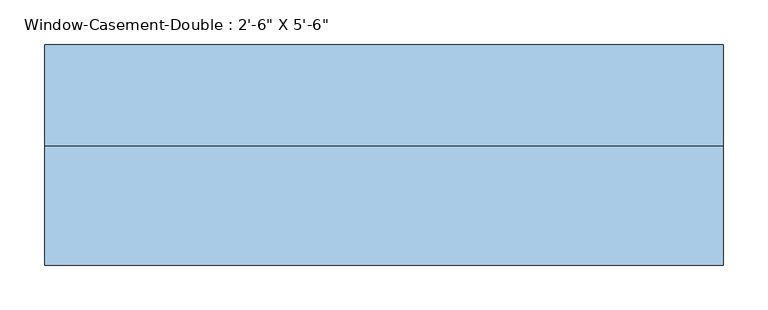
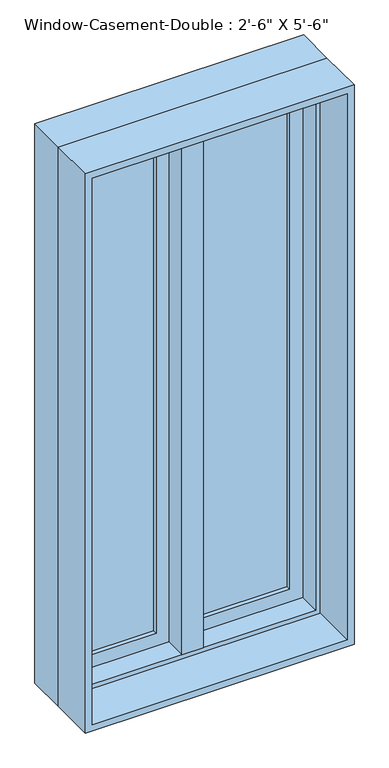
"""IFC4 building model written with IfcOpenShell, lengths in millimetres: window geometry."""

from ifc_helpers import new_model, si_unit, frame, origin, place, context, project, spatial, polyline, outline, extrude, faceted_brep, source, transform, mapped, element, save


def window_9dcce3b5(model_context):
    return source(origin(), model_context, "Body", "SolidModel", [
        faceted_brep([(9.525, 133.35, 2578.1), (-9.525, 133.35, 2578.1), (-9.525, 82.55, 2578.1), (9.525, 82.55, 2578.1), (9.525, 133.35, 927.1), (9.525, 82.55, 927.1), (-9.525, 82.55, 927.1), (-9.525, 133.35, 927.1), (-9.525, 82.55, 946.15), (-9.525, 82.55, 2559.05), (-30.1625, 82.55, 946.15), (-30.1625, 82.55, 2559.05), (-30.1625, 19.05, 946.15), (-30.1625, 19.05, 2559.05), (30.1625, 19.05, 946.15), (30.1625, 19.05, 2559.05), (30.1625, 82.55, 946.15), (30.1625, 82.55, 2559.05), (9.525, 82.55, 946.15), (9.525, 82.55, 2559.05)], [[[0, 1, 2, 3]], [[4, 5, 6, 7]], [[1, 0, 4, 7]], [[2, 1, 7, 6, 8, 9]], [[9, 8, 10, 11]], [[11, 10, 12, 13]], [[13, 12, 14, 15]], [[15, 14, 16, 17]], [[17, 16, 18, 19]], [[0, 3, 19, 18, 5, 4]], [[18, 8, 6, 5]], [[9, 19, 3, 2]], [[8, 18, 16, 14, 12, 10]], [[19, 9, 11, 13, 15, 17]]]),
        extrude(outline(polyline([(-66.675, 114.3), (-66.675, 107.95), (-311.15, 107.95), (-311.15, 114.3), (-66.675, 114.3)])), frame((0.0, 0.0, 984.25), z_axis=(0.0, 0.0, 1.0), x_axis=(1.0, 0.0, 0.0)), (0.0, 0.0, 1.0), 1536.7),
        extrude(outline(polyline([(-311.15, 95.25), (-311.15, 101.6), (-66.675, 101.6), (-66.675, 95.25), (-311.15, 95.25)])), frame((0.0, 0.0, 984.25), z_axis=(0.0, 0.0, 1.0), x_axis=(1.0, 0.0, 0.0)), (0.0, 0.0, 1.0), 1536.7),
        extrude(outline(polyline([(311.15, 114.3), (311.15, 107.95), (66.675, 107.95), (66.675, 114.3), (311.15, 114.3)])), frame((0.0, 0.0, 984.25), z_axis=(0.0, 0.0, 1.0), x_axis=(1.0, 0.0, 0.0)), (0.0, 0.0, 1.0), 1536.7),
        extrude(outline(polyline([(66.675, 95.25), (66.675, 101.6), (311.15, 101.6), (311.15, 95.25), (66.675, 95.25)])), frame((0.0, 0.0, 984.25), z_axis=(0.0, 0.0, 1.0), x_axis=(1.0, 0.0, 0.0)), (0.0, 0.0, 1.0), 1536.7),
        extrude(outline(polyline([(2578.1, -368.3), (927.1, -368.3), (927.1, -9.525), (2578.1, -9.525), (2578.1, -368.3)]), holes=[polyline([(2520.95, -66.675), (984.25, -66.675), (984.25, -311.15), (2520.95, -311.15), (2520.95, -66.675)])]), frame((0.0, 82.55, 0.0), z_axis=(0.0, 1.0, 0.0), x_axis=(0.0, 0.0, 1.0)), (0.0, 0.0, 1.0), 44.45),
        extrude(outline(polyline([(927.1, 368.3), (2578.1, 368.3), (2578.1, 9.525), (927.1, 9.525), (927.1, 368.3)]), holes=[polyline([(984.25, 66.675), (2520.95, 66.675), (2520.95, 311.15), (984.25, 311.15), (984.25, 66.675)])]), frame((0.0, 82.55, 0.0), z_axis=(0.0, 1.0, 0.0), x_axis=(0.0, 0.0, 1.0)), (0.0, 0.0, 1.0), 44.45),
        extrude(outline(polyline([(2590.8, -381.0), (914.4, -381.0), (914.4, 381.0), (2590.8, 381.0), (2590.8, -381.0)]), holes=[polyline([(2571.75, 361.95), (933.45, 361.95), (933.45, -361.95), (2571.75, -361.95), (2571.75, 361.95)])]), frame((0.0, -114.3, 0.0), z_axis=(0.0, 1.0, 0.0), x_axis=(0.0, 0.0, 1.0)), (0.0, 0.0, 1.0), 133.35),
        faceted_brep([(349.25, 82.55, 2559.05), (349.25, 19.05, 2559.05), (-349.25, 19.05, 2559.05), (-349.25, 82.55, 2559.05), (368.3, 133.35, 2578.1), (368.3, 82.55, 2578.1), (-368.3, 82.55, 2578.1), (-368.3, 133.35, 2578.1), (381.0, 19.05, 2590.8), (381.0, 133.35, 2590.8), (-381.0, 133.35, 2590.8), (-381.0, 19.05, 2590.8), (-349.25, 19.05, 946.15), (-349.25, 82.55, 946.15), (-368.3, 82.55, 927.1), (-368.3, 133.35, 927.1), (-381.0, 133.35, 914.4), (-381.0, 19.05, 914.4), (349.25, 19.05, 946.15), (349.25, 82.55, 946.15), (368.3, 82.55, 927.1), (368.3, 133.35, 927.1), (381.0, 133.35, 914.4), (381.0, 19.05, 914.4)], [[[0, 1, 2, 3]], [[4, 5, 6, 7]], [[8, 9, 10, 11]], [[3, 2, 12, 13]], [[7, 6, 14, 15]], [[11, 10, 16, 17]], [[13, 12, 18, 19]], [[15, 14, 20, 21]], [[17, 16, 22, 23]], [[11, 17, 23, 8], [1, 18, 12, 2]], [[19, 18, 1, 0]], [[5, 20, 14, 6], [3, 13, 19, 0]], [[21, 20, 5, 4]], [[23, 22, 9, 8]], [[9, 22, 16, 10], [7, 15, 21, 4]]]),
    ])


if __name__ == "__main__":
    model = new_model("IFC4")
    model_context = context("Model", 3, world=origin())
    ifc_project = project(units=[si_unit("LENGTHUNIT", "METRE", prefix="MILLI")], contexts=[model_context])
    site = spatial("IfcSite", under=ifc_project)
    building = spatial("IfcBuilding", under=site)
    placement = place(None, origin())
    window_shape = window_9dcce3b5(model_context)
    element("IfcWindow", 1, ObjectType="Window-Casement-Double : 2'-6\" X 5'-6\"", at=placement, inside=building, context=model_context, shape_type="MappedRepresentation", body=[
        mapped(window_shape, transform((0.0, 0.0, 0.0), x_axis=(1.0, 0.0, 0.0), y_axis=(0.0, 1.0, 0.0), z_axis=(0.0, 0.0, 1.0))),
    ])
    save(model, "model.ifc")

# Revit data of these elements
# Type "Window-Casement-Double : 2'-6\" X 5'-6\""
#   Type Mark = "21"
#   Fire Rating = "0.5h"
#   Assembly Code = "B2020100"
#   Analytic Construction = "Double glazing - domestic"
#   Frame Extension [instance default] = 0' - 0 1/4"
#   Window Inset [instance default] = 0' - 0"
#   Wall Thickness [instance default] = 0' - 6"
#   Interior Wall Closure [instance default] = 0' - 2 1/4"
#   Half Width = 1' - 3"
#   Visual Light Transmittance = 0.81
#   Thermal Resistance (R) = 1.8146 (h·ft²·°F)/BTU
#   Solar Heat Gain Coefficient = 0.76
#   Rough Width = 2' - 6 1/2"
#   Rough Height = 5' - 6 1/2"
#   Height = 5' - 6"
#   Heat Transfer Coefficient (U) = 0.5511 BTU/(h·ft²·°F)
#   Exterior Wall Closure [instance default] = 0' - 1 1/4"
#   Extension Jamb [instance default] = 0' - 2 1/4"
#   Default Sill Height = 3' - 0"
#   Width = 2' - 6"
#   Muntin Visibility = yes
#   Interior Trim Visibility [instance default] = yes
#   Exterior Trim Visibility [instance default] = yes
#   Extension Jamb Visibility [instance default] = yes
#   Interior Trim Material = Wood - Stained
#   Muntin Pattern = Muntin Pattern_2x2 : Muntin Pattern_2x2
#   Interior Trim = Trim-Window-Interior-Flat : Picture Frame
#   Interior Frame Material = Wood - Stained
#   Glass Panel Material = Glass
#   Exterior Trim Material = Clad - White
#   Exterior Trim = Trim-Window-Exterior-Flat : with Sill
#   Exterior Frame Material = Clad - White
#   Wall Closure = (empty or 0)
# Element 1 (IfcWindow, "Window-Casement-Double : 2'-6\" X 5'-6\"")
#   Wall Thickness = 0' - 9"
#   Extension Jamb = 0' - 5 1/4"
#   Materials on its faces: "Wood - Stained", "Glass", "Clad - White"
# Materials
#   "Wood - Stained": class "Wood", colour RGB 224 178 126, transparency 0, Cost = 0
#   "Glass": class "Glass", colour RGB 0 128 192, transparency 0.75, Description = "Soda Lime Glass", Cost = 0
#   "Clad - White": class "Wood", colour RGB 242 242 238, transparency 0, Cost = 0
